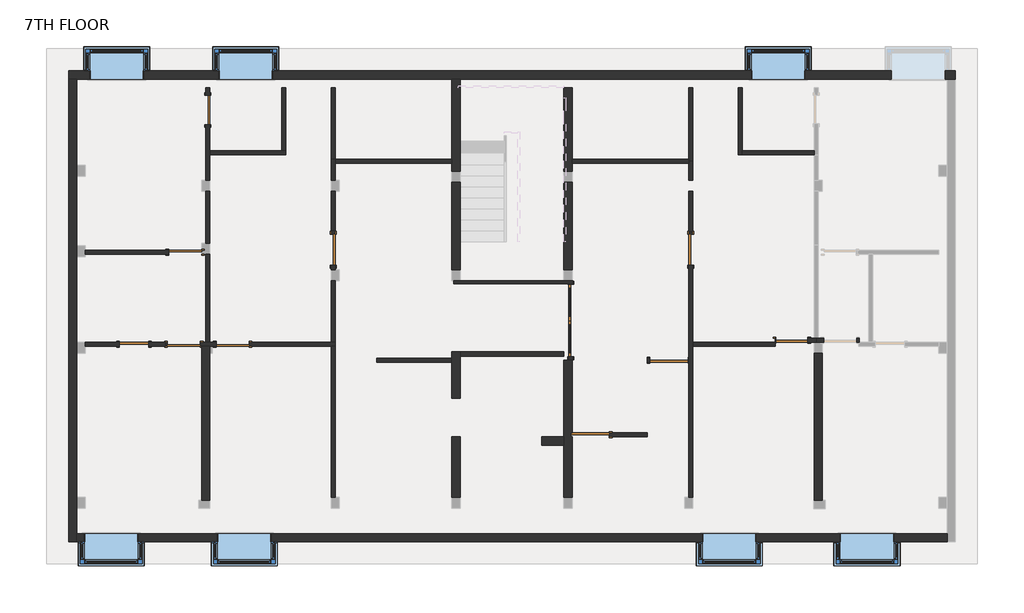
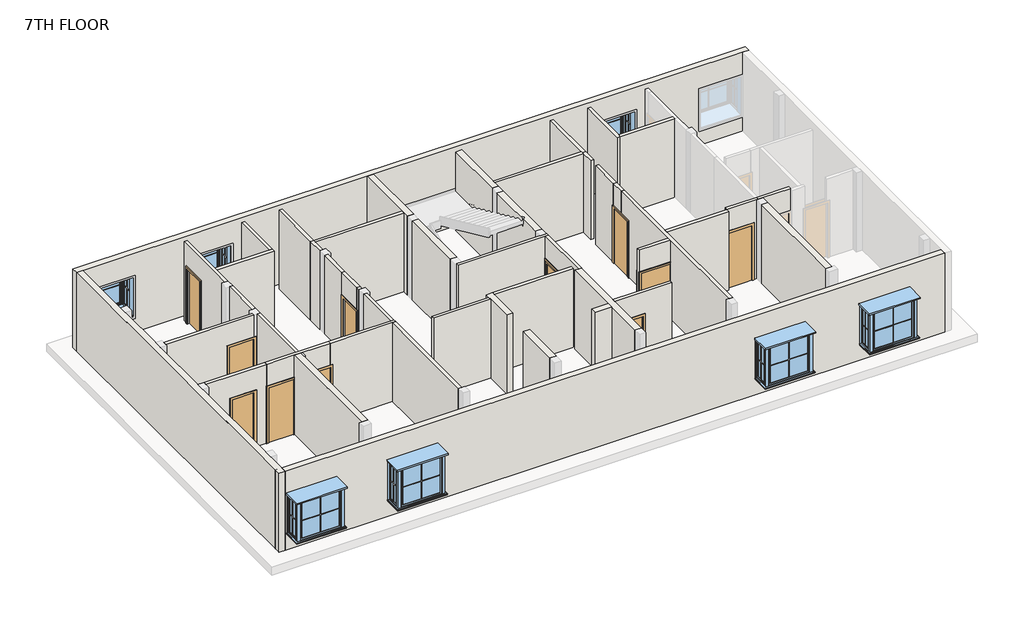
# One storey, part 1 of 2: 48 walls, 11 doors, 7 windows.
"""IFC4 building model written with IfcOpenShell, lengths in millimetres."""

from ifc_helpers import new_model, si_unit, frame, origin, place, context, project, spatial, polyline, outline, extrude, faceted_brep, transform, mapped, element, save
from components import door_04ab2522, m_door_single_panel_05506f71, door_07b5d71c, door_85b31ab1, door_1991e9a2, door_4c0a2014, door_82def9da, m_door_single_panel_3_x7_f8176753, m_door_single_panel_3_x7_ebb67e73, window_19bbd869

model = new_model("IFC4")

# Units and contexts
model_context = context("Model", 3, world=origin())
ifc_project = project(units=[si_unit("LENGTHUNIT", "METRE", prefix="MILLI")], contexts=[model_context])

# Site, building, storey
site = spatial("IfcSite", under=ifc_project)
building = spatial("IfcBuilding", under=site)
storey = spatial("IfcBuildingStorey", under=building, Name="7TH FLOOR", Elevation=25603.2)

# Doors
placement = place(None, origin())
door_shape = door_04ab2522(model_context)
element("IfcDoor", 1, ObjectType="M_Door-Double-Glass : 6'7\"X7'", at=placement, inside=storey, context=model_context, shape_type="MappedRepresentation", body=[
    mapped(door_shape, transform((1217.5394962, 1183.3817656, 25603.2), x_axis=(0.0, 1.0, 0.0), y_axis=(-1.0, 0.0, 0.0), z_axis=(0.0, 0.0, 1.0))),
])
m_door_single_panel_shape = m_door_single_panel_05506f71(model_context)
element("IfcDoor", 2, ObjectType="M_Door-Single-Panel", at=placement, inside=storey, context=model_context, shape_type="MappedRepresentation", body=[
    mapped(m_door_single_panel_shape, transform((1745.3012085, -1975.7432663, 25603.2), x_axis=(-1.0, 0.0, 0.0), y_axis=(0.0, -1.0, 0.0), z_axis=(0.0, 0.0, 1.0))),
])
element("IfcDoor", 3, ObjectType="M_Door-Single-Panel", at=placement, inside=storey, context=model_context, shape_type="MappedRepresentation", body=[
    mapped(m_door_single_panel_shape, transform((3933.4813133, 90.9578621, 25603.2), x_axis=(1.0, 0.0, 0.0), y_axis=(0.0, 1.0, 0.0), z_axis=(0.0, 0.0, 1.0))),
])
door_2_shape = door_07b5d71c(model_context)
element("IfcDoor", 4, ObjectType="M_Door-Single-Panel : 2'10\"X7' 2", at=placement, inside=storey, context=model_context, shape_type="MappedRepresentation", body=[
    mapped(door_2_shape, transform((-5360.3487995, 3142.9626891, 25603.2), x_axis=(0.0, -1.0, 0.0), y_axis=(1.0, 0.0, 0.0), z_axis=(0.0, 0.0, 1.0))),
])
door_3_shape = door_85b31ab1(model_context)
element("IfcDoor", 5, ObjectType="M_Door-Single-Panel : 2'10\"X7' 2", at=placement, inside=storey, context=model_context, shape_type="MappedRepresentation", body=[
    mapped(door_3_shape, transform((4532.9512082, 3142.9626891, 25603.2), x_axis=(0.0, -1.0, 0.0), y_axis=(1.0, 0.0, 0.0), z_axis=(0.0, 0.0, 1.0))),
])
door_4_shape = door_1991e9a2(model_context)
element("IfcDoor", 6, ObjectType="M_Door-Single-Panel : 2'11\"X7' 3", at=placement, inside=storey, context=model_context, shape_type="MappedRepresentation", body=[
    mapped(door_4_shape, transform((7330.1405552, 640.4567334, 25603.2), x_axis=(1.0, 0.0, 0.0), y_axis=(0.0, 1.0, 0.0), z_axis=(0.0, 0.0, 1.0))),
])
door_5_shape = door_4c0a2014(model_context)
element("IfcDoor", 7, ObjectType="M_Door-Single-Panel : 2'8\"X7'", at=placement, inside=storey, context=model_context, shape_type="MappedRepresentation", body=[
    mapped(door_5_shape, transform((-10873.4462614, 526.1567334, 25603.2), x_axis=(1.0, 0.0, 0.0), y_axis=(0.0, 1.0, 0.0), z_axis=(0.0, 0.0, 1.0))),
])
door_6_shape = door_82def9da(model_context)
element("IfcDoor", 8, ObjectType="M_Door-Single-Panel : 2'8\"X7'", at=placement, inside=storey, context=model_context, shape_type="MappedRepresentation", body=[
    mapped(door_6_shape, transform((-8827.4487992, 7008.6751452, 25603.2), x_axis=(0.0, 1.0, 0.0), y_axis=(-1.0, 0.0, 0.0), z_axis=(0.0, 0.0, 1.0))),
])
m_door_single_panel_3_x7_shape = m_door_single_panel_3_x7_f8176753(model_context)
element("IfcDoor", 9, ObjectType="M_Door-Single-Panel : 3'X7'", at=placement, inside=storey, context=model_context, shape_type="MappedRepresentation", body=[
    mapped(m_door_single_panel_3_x7_shape, transform((-9456.0987989, 3078.8567332, 25603.2), x_axis=(1.0, 0.0, 0.0), y_axis=(0.0, 1.0, 0.0), z_axis=(0.0, 0.0, 1.0))),
])
element("IfcDoor", 10, ObjectType="M_Door-Single-Panel : 3'X7'", at=placement, inside=storey, context=model_context, shape_type="MappedRepresentation", body=[
    mapped(m_door_single_panel_3_x7_shape, transform((-8144.8381465, 526.1567334, 25603.2), x_axis=(-1.0, 0.0, 0.0), y_axis=(0.0, -1.0, 0.0), z_axis=(0.0, 0.0, 1.0))),
])
m_door_single_panel_3_x7_2_shape = m_door_single_panel_3_x7_ebb67e73(model_context)
element("IfcDoor", 11, ObjectType="M_Door-Single-Panel : 3'X7'", at=placement, inside=storey, context=model_context, shape_type="MappedRepresentation", body=[
    mapped(m_door_single_panel_3_x7_2_shape, transform((-9494.1987992, 526.1567334, 25603.2), x_axis=(1.0, 0.0, 0.0), y_axis=(0.0, 1.0, 0.0), z_axis=(0.0, 0.0, 1.0))),
])

# Walls
element("IfcWall", 12, ObjectType="3.5\"", at=placement, inside=storey, context=model_context, shape_type="Brep", body=[
    faceted_brep([(-2020.2487998, 2196.2067742, 25603.2), (1158.0082462, 2196.2067742, 25603.2), (1272.3082462, 2196.2067742, 25603.2), (1272.3082462, 2196.2067742, 28651.2), (1158.0082462, 2196.2067742, 28651.2), (-2020.2487998, 2196.2067742, 28651.2), (-2020.2487998, 2285.1067742, 25603.2), (-2020.2487998, 2285.1067742, 28651.2), (-1845.5417538, 2285.1067742, 28651.2), (1024.6582462, 2285.1067742, 28651.2), (1253.2582462, 2285.1067742, 28651.2), (1272.3082462, 2285.1067742, 28651.2), (1272.3082462, 2285.1067742, 25603.2), (1253.2582462, 2285.1067742, 25603.2), (1024.6582462, 2285.1067742, 25603.2), (-1845.5417538, 2285.1067742, 25603.2)], [[[0, 1, 2, 3, 4, 5]], [[6, 7, 8, 9, 10, 11, 12, 13, 14, 15]], [[2, 1, 0, 6, 15, 14, 13, 12]], [[5, 4, 3, 11, 10, 9, 8, 7]], [[0, 5, 7, 6]], [[3, 2, 12, 11]]]),
])
element("IfcWall", 13, ObjectType="4.5\"", at=placement, inside=storey, context=model_context, shape_type="SweptSolid", body=[
    extrude(outline(polyline([(3132.0737955, 28651.2), (3628.3344162, 28651.2), (3628.3344162, 25603.2), (3574.7626891, 25603.2), (3574.7626891, 27736.8), (3132.0737955, 27736.8), (3132.0737955, 28651.2)])), frame((4475.8012082, 0.0, 0.0), z_axis=(1.0, 0.0, 0.0), x_axis=(0.0, 1.0, 0.0)), (0.0, 0.0, 1.0), 114.3),
])
element("IfcWall", 14, ObjectType="4.5\"", at=placement, inside=storey, context=model_context, shape_type="SweptSolid", body=[
    extrude(outline(polyline([(2711.1626891, 28651.2), (3671.8272228, 28651.2), (3671.8272228, 25603.2), (3574.7626891, 25603.2), (3574.7626891, 27736.8), (2711.1626891, 27736.8), (2711.1626891, 28651.2)])), frame((-5417.4987995, 0.0, 0.0), z_axis=(1.0, 0.0, 0.0), x_axis=(0.0, 1.0, 0.0)), (0.0, 0.0, 1.0), 114.3),
])
element("IfcWall", 15, ObjectType="4.5\"", at=placement, inside=storey, context=model_context, shape_type="Brep", body=[
    faceted_brep([(-7690.1644155, 469.0067334, 28651.2), (-8713.148796, 469.0067334, 28651.2), (-8771.750543, 469.0067334, 28651.2), (-9000.350543, 469.0067334, 28651.2), (-10009.8462614, 469.0067334, 28651.2), (-10009.8462614, 469.0067334, 25603.2), (-9951.3987992, 469.0067334, 25603.2), (-9951.3987992, 469.0067334, 27736.8), (-9036.9987992, 469.0067334, 27736.8), (-9036.9987992, 469.0067334, 25603.2), (-9000.350543, 469.0067334, 25603.2), (-8771.750543, 469.0067334, 25603.2), (-8713.148796, 469.0067334, 25603.2), (-8602.0381465, 469.0067334, 25603.2), (-8602.0381465, 469.0067334, 27736.8), (-7690.1644155, 469.0067334, 27736.8), (-10009.8462614, 583.3067334, 28651.2), (-7690.1644155, 583.3067334, 28651.2), (-7690.1644155, 583.3067334, 27736.8), (-8602.0381465, 583.3067334, 27736.8), (-8602.0381465, 583.3067334, 25603.2), (-9036.9987992, 583.3067334, 25603.2), (-9036.9987992, 583.3067334, 27736.8), (-9951.3987992, 583.3067334, 27736.8), (-9951.3987992, 583.3067334, 25603.2), (-10009.8462614, 583.3067334, 25603.2)], [[[0, 1, 2, 3, 4, 5, 6, 7, 8, 9, 10, 11, 12, 13, 14, 15]], [[16, 17, 18, 19, 20, 21, 22, 23, 24, 25]], [[5, 25, 24, 6]], [[9, 21, 20, 13, 12, 11, 10]], [[17, 0, 15, 18]], [[4, 3, 2, 1, 0, 17, 16]], [[5, 4, 16, 25]], [[8, 22, 21, 9]], [[7, 23, 22, 8]], [[23, 7, 6, 24]], [[19, 14, 13, 20]], [[14, 19, 18, 15]]]),
])
element("IfcWall", 16, ObjectType="4.5\"", at=placement, inside=storey, context=model_context, shape_type="Brep", body=[
    faceted_brep([(8000.0512079, 583.3067334, 25603.2), (8000.0512079, 583.3067334, 28651.2), (7942.9012047, 583.3067334, 28651.2), (6862.7668241, 583.3067334, 28651.2), (6862.7668241, 583.3067334, 25603.2), (6885.6405552, 583.3067334, 25603.2), (6885.6405552, 583.3067334, 27736.8), (7774.6405552, 583.3067334, 27736.8), (7774.6405552, 583.3067334, 25603.2), (7942.9012047, 583.3067334, 25603.2), (8000.0512079, 697.6067334, 28651.2), (8000.0512079, 697.6067334, 25603.2), (7942.9012079, 697.6067334, 25603.2), (7774.6405552, 697.6067334, 25603.2), (7774.6405552, 697.6067334, 27736.8), (6885.6405552, 697.6067334, 27736.8), (6885.6405552, 697.6067334, 25603.2), (6862.7668241, 697.6067334, 25603.2), (6862.7668241, 697.6067334, 28651.2), (7942.9012079, 697.6067334, 28651.2)], [[[0, 1, 2, 3, 4, 5, 6, 7, 8, 9]], [[10, 11, 12, 13, 14, 15, 16, 17, 18, 19]], [[4, 17, 16, 5]], [[11, 0, 9, 8, 13, 12]], [[1, 0, 11, 10]], [[3, 2, 1, 10, 19, 18]], [[4, 3, 18, 17]], [[7, 14, 13, 8]], [[14, 7, 6, 15]], [[15, 6, 5, 16]]]),
])
element("IfcWall", 17, ObjectType="4.5\"", at=placement, inside=storey, context=model_context, shape_type="Brep", body=[
    faceted_brep([(9187.5012047, 583.3067334, 25603.2), (9187.5012047, 583.3067334, 28651.2), (8171.5012047, 583.3067334, 28651.2), (8000.0512079, 583.3067334, 28651.2), (8000.0512079, 583.3067334, 25603.2), (8171.5012047, 583.3067334, 25603.2), (8209.6012079, 583.3067334, 25603.2), (8209.6012079, 583.3067334, 27736.8), (9124.0012079, 583.3067334, 27736.8), (9124.0012079, 583.3067334, 25603.2), (9187.5012047, 697.6067334, 28651.2), (9187.5012047, 697.6067334, 25603.2), (9124.0012079, 697.6067334, 25603.2), (9124.0012079, 697.6067334, 27736.8), (8209.6012079, 697.6067334, 27736.8), (8209.6012079, 697.6067334, 25603.2), (8057.2012079, 697.6067334, 25603.2), (8000.0512079, 697.6067334, 25603.2), (8000.0512079, 697.6067334, 28651.2), (8057.2012079, 697.6067334, 28651.2)], [[[0, 1, 2, 3, 4, 5, 6, 7, 8, 9]], [[10, 11, 12, 13, 14, 15, 16, 17, 18, 19]], [[11, 0, 9, 12]], [[4, 17, 16, 15, 6, 5]], [[1, 0, 11, 10]], [[3, 2, 1, 10, 19, 18]], [[4, 3, 18, 17]], [[7, 14, 13, 8]], [[8, 13, 12, 9]], [[14, 7, 6, 15]]]),
])
element("IfcWall", 18, ObjectType="4.5\"", at=placement, inside=storey, context=model_context, shape_type="SweptSolid", body=[
    extrude(outline(polyline([(25603.2, 3334.0114184), (28651.2, 3334.0114184), (28651.2, 1250.0012085), (27736.8, 1250.0012085), (27736.8, 2278.7012085), (25603.2, 2278.7012085), (25603.2, 3334.0114184)])), frame((0.0, -2032.8932663, 0.0), z_axis=(0.0, 1.0, 0.0), x_axis=(0.0, 0.0, 1.0)), (0.0, 0.0, 1.0), 114.3),
])
element("IfcWall", 19, ObjectType="4.5\"", at=placement, inside=storey, context=model_context, shape_type="SweptSolid", body=[
    extrude(outline(polyline([(27736.8, 4466.8813133), (25603.2, 4466.8813133), (25603.2, 4475.8012082), (28651.2, 4475.8012082), (28651.2, 3334.0114184), (25603.2, 3334.0114184), (25603.2, 3400.0813133), (27736.8, 3400.0813133), (27736.8, 4466.8813133)])), frame((0.0, 33.8078621, 0.0), z_axis=(0.0, 1.0, 0.0), x_axis=(0.0, 0.0, 1.0)), (0.0, 0.0, 1.0), 114.3),
])
element("IfcWall", 20, ObjectType="4.5\"", at=placement, inside=storey, context=model_context, shape_type="SweptSolid", body=[
    extrude(outline(polyline([(1021.4012085, 202.3067742), (-1848.7987998, 202.3067742), (-1848.7987998, 316.6067742), (1021.4012085, 316.6067742), (1021.4012085, 202.3067742)])), frame((0.0, 0.0, 25603.2), z_axis=(0.0, 0.0, 1.0), x_axis=(1.0, 0.0, 0.0)), (0.0, 0.0, 1.0), 3048.0),
])
element("IfcWall", 21, ObjectType="4.5\"", at=placement, inside=storey, context=model_context, shape_type="Brep", body=[
    faceted_brep([(1158.0082462, 2196.2067742, 25603.2), (1158.0082462, 2186.6817656, 25603.2), (1158.0082462, 2186.6817656, 27736.8), (1158.0082462, 180.0817656, 27736.8), (1158.0082462, 180.0817656, 25603.2), (1158.0082462, 90.9578621, 25603.2), (1158.0082462, 90.9578621, 28651.2), (1158.0082462, 2196.2067742, 28651.2), (1272.3082462, 2186.6817656, 27736.8), (1272.3082462, 2186.6817656, 25603.2), (1272.3082462, 2196.2067742, 25603.2), (1272.3082462, 2196.2067742, 28651.2), (1272.3082462, 90.9578621, 28651.2), (1272.3082462, 90.9578621, 25603.2), (1272.3082462, 180.0817656, 25603.2), (1272.3082462, 180.0817656, 27736.8), (1250.0012085, 90.9578621, 25603.2), (1250.0012085, 90.9578621, 28651.2)], [[[0, 1, 2, 3, 4, 5, 6, 7]], [[8, 9, 10, 11, 12, 13, 14, 15]], [[14, 13, 16, 5, 4]], [[10, 9, 1, 0]], [[6, 5, 16, 13, 12, 17]], [[7, 6, 17, 12, 11]], [[0, 7, 11, 10]], [[2, 1, 9, 8]], [[3, 2, 8, 15]], [[4, 3, 15, 14]]]),
])
element("IfcWall", 22, ObjectType="4.5\"", at=placement, inside=storey, context=model_context, shape_type="Brep", body=[
    faceted_brep([(1250.0012085, 5536.3067329, 25603.2), (4475.8012082, 5536.3067329, 25603.2), (4475.8012082, 5536.3067329, 28651.2), (1250.0012085, 5536.3067329, 28651.2), (1250.0012085, 5650.6067329, 25603.2), (1250.0012085, 5650.6067329, 28651.2), (4475.8012082, 5650.6067329, 28651.2), (4475.8012082, 5650.6067329, 25603.2), (4475.8012082, 5593.4567329, 25603.2), (4475.8012082, 5593.4567329, 28651.2)], [[[0, 1, 2, 3]], [[4, 5, 6, 7]], [[1, 0, 4, 7, 8]], [[3, 2, 9, 6, 5]], [[2, 1, 8, 7, 6, 9]], [[0, 3, 5, 4]]]),
])
element("IfcWall", 23, ObjectType="4.5\"", at=placement, inside=storey, context=model_context, shape_type="SweptSolid", body=[
    extrude(outline(polyline([(-5417.4987995, -3709.2932193), (-5417.4987995, 469.0067334), (-5303.1987995, 469.0067334), (-5303.1987995, -3709.2932193), (-5417.4987995, -3709.2932193)])), frame((0.0, 0.0, 25603.2), z_axis=(0.0, 0.0, 1.0), x_axis=(1.0, 0.0, 0.0)), (0.0, 0.0, 1.0), 3048.0),
])
element("IfcWall", 24, ObjectType="4.5\" 2", at=placement, inside=storey, context=model_context, shape_type="SweptSolid", body=[
    extrude(outline(polyline([(28651.2, -8998.8987989), (28651.2, -12224.6987989), (25603.2, -12224.6987989), (25603.2, -9913.2987989), (27736.8, -9913.2987989), (27736.8, -8998.8987989), (28651.2, -8998.8987989)])), frame((0.0, 3021.7067332, 0.0), z_axis=(0.0, 1.0, 0.0), x_axis=(0.0, 0.0, 1.0)), (0.0, 0.0, 1.0), 114.3),
])
element("IfcWall", 25, ObjectType="4.5\" 2", at=placement, inside=storey, context=model_context, shape_type="SweptSolid", body=[
    extrude(outline(polyline([(-8770.2987992, 4761.606733), (-8770.2987992, 3326.5067332), (-8884.5987992, 3326.5067332), (-8884.5987992, 4761.606733), (-8770.2987992, 4761.606733)])), frame((0.0, 0.0, 25603.2), z_axis=(0.0, 0.0, 1.0), x_axis=(1.0, 0.0, 0.0)), (0.0, 0.0, 1.0), 3048.0),
])
element("IfcWall", 26, ObjectType="4.5\" 2", at=placement, inside=storey, context=model_context, shape_type="Brep", body=[
    faceted_brep([(-8770.2987992, 7415.0751452, 27736.8), (-8770.2987992, 7415.0751452, 25603.2), (-8770.2987992, 7631.8067329, 25603.2), (-8770.2987992, 7631.8067329, 28651.2), (-8770.2987992, 5879.2067329, 28651.2), (-8770.2987992, 5764.9067329, 28651.2), (-8770.2987992, 5066.406733, 28651.2), (-8770.2987992, 5066.406733, 25603.2), (-8770.2987992, 5764.9067329, 25603.2), (-8770.2987992, 5879.2067329, 25603.2), (-8770.2987992, 6602.2751452, 25603.2), (-8770.2987992, 6602.2751452, 27736.8), (-8884.5987992, 7631.8067329, 25603.2), (-8884.5987992, 7415.0751452, 25603.2), (-8884.5987992, 7415.0751452, 27736.8), (-8884.5987992, 6602.2751452, 27736.8), (-8884.5987992, 6602.2751452, 25603.2), (-8884.5987992, 5066.406733, 25603.2), (-8884.5987992, 5066.406733, 28651.2), (-8884.5987992, 7631.8067329, 28651.2)], [[[0, 1, 2, 3, 4, 5, 6, 7, 8, 9, 10, 11]], [[12, 13, 14, 15, 16, 17, 18, 19]], [[2, 1, 13, 12]], [[10, 9, 8, 7, 17, 16]], [[3, 2, 12, 19]], [[6, 5, 4, 3, 19, 18]], [[7, 6, 18, 17]], [[14, 13, 1, 0]], [[15, 14, 0, 11]], [[16, 15, 11, 10]]]),
])
element("IfcWall", 27, ObjectType="4.5\" 2", at=placement, inside=storey, context=model_context, shape_type="Brep", body=[
    faceted_brep([(-8770.2987992, 5764.9067329, 25603.2), (-6674.7987994, 5764.9067329, 25603.2), (-6674.7987994, 5764.9067329, 28651.2), (-8770.2987992, 5764.9067329, 28651.2), (-8770.2987992, 5879.2067329, 25603.2), (-8770.2987992, 5879.2067329, 28651.2), (-6789.0987994, 5879.2067329, 28651.2), (-6674.7987994, 5879.2067329, 28651.2), (-6674.7987994, 5879.2067329, 25603.2), (-6789.0987994, 5879.2067329, 25603.2)], [[[0, 1, 2, 3]], [[4, 5, 6, 7, 8, 9]], [[1, 0, 4, 9, 8]], [[3, 2, 7, 6, 5]], [[0, 3, 5, 4]], [[2, 1, 8, 7]]]),
])
element("IfcWall", 28, ObjectType="4.5\" 2", at=placement, inside=storey, context=model_context, shape_type="SweptSolid", body=[
    extrude(outline(polyline([(-6674.7987994, 7631.8067329), (-6674.7987994, 5879.2067329), (-6789.0987994, 5879.2067329), (-6789.0987994, 7631.8067329), (-6674.7987994, 7631.8067329)])), frame((0.0, 0.0, 25603.2), z_axis=(0.0, 0.0, 1.0), x_axis=(1.0, 0.0, 0.0)), (0.0, 0.0, 1.0), 3048.0),
])
element("IfcWall", 29, ObjectType="4.5\" 2", at=placement, inside=storey, context=model_context, shape_type="SweptSolid", body=[
    extrude(outline(polyline([(27736.8, -10467.0462614), (25603.2, -10467.0462614), (25603.2, -10009.8462614), (28651.2, -10009.8462614), (28651.2, -12224.6987989), (25603.2, -12224.6987989), (25603.2, -11279.8462614), (27736.8, -11279.8462614), (27736.8, -10467.0462614)])), frame((0.0, 469.0067334, 0.0), z_axis=(0.0, 1.0, 0.0), x_axis=(0.0, 0.0, 1.0)), (0.0, 0.0, 1.0), 114.3),
])
element("IfcWall", 30, ObjectType="4.5\" 2", at=placement, inside=storey, context=model_context, shape_type="SweptSolid", body=[
    extrude(outline(polyline([(-8770.298796, 3021.7067332), (-8770.298796, 583.3067804), (-8884.598796, 583.3067804), (-8884.598796, 3021.7067332), (-8770.298796, 3021.7067332)])), frame((0.0, 0.0, 25603.2), z_axis=(0.0, 0.0, 1.0), x_axis=(1.0, 0.0, 0.0)), (0.0, 0.0, 1.0), 3048.0),
])
element("IfcWall", 31, ObjectType="4.5\" 2", at=placement, inside=storey, context=model_context, shape_type="Brep", body=[
    faceted_brep([(-5303.1987995, 469.0067334, 28651.2), (-5417.4987995, 469.0067334, 28651.2), (-7690.1644155, 469.0067334, 28651.2), (-7690.1644155, 469.0067334, 27736.8), (-7687.6381465, 469.0067334, 27736.8), (-7687.6381465, 469.0067334, 25603.2), (-5417.4987995, 469.0067334, 25603.2), (-5303.1987995, 469.0067334, 25603.2), (-7690.1644155, 583.3067334, 28651.2), (-5417.4987995, 583.3067334, 28651.2), (-5303.1987995, 583.3067334, 28651.2), (-5303.1987995, 583.3067334, 25603.2), (-5417.4987995, 583.3067334, 25603.2), (-7687.6381465, 583.3067334, 25603.2), (-7687.6381465, 583.3067334, 27736.8), (-7690.1644155, 583.3067334, 27736.8)], [[[0, 1, 2, 3, 4, 5, 6, 7]], [[8, 9, 10, 11, 12, 13, 14, 15]], [[11, 7, 6, 5, 13, 12]], [[2, 1, 0, 10, 9, 8]], [[2, 8, 15, 3]], [[0, 7, 11, 10]], [[14, 4, 3, 15]], [[4, 14, 13, 5]]]),
])
element("IfcWall", 32, ObjectType="4.5\" 2", at=placement, inside=storey, context=model_context, shape_type="SweptSolid", body=[
    extrude(outline(polyline([(-5303.1987995, 2285.1067802), (-5303.1987995, 583.3067334), (-5417.4987995, 583.3067334), (-5417.4987995, 2285.1067802), (-5303.1987995, 2285.1067802)])), frame((0.0, 0.0, 25603.2), z_axis=(0.0, 0.0, 1.0), x_axis=(1.0, 0.0, 0.0)), (0.0, 0.0, 1.0), 3048.0),
])
element("IfcWall", 33, ObjectType="4.5\" 2", at=placement, inside=storey, context=model_context, shape_type="Brep", body=[
    faceted_brep([(-5303.1987995, 2589.9067802, 25603.2), (-5303.1987995, 2711.1626891, 25603.2), (-5303.1987995, 2711.1626891, 27736.8), (-5303.1987995, 2711.1626891, 28651.2), (-5303.1987995, 2589.9067802, 28651.2), (-5417.4987995, 2589.9067802, 25603.2), (-5417.4987995, 2589.9067802, 28651.2), (-5417.4987995, 2711.1626891, 28651.2), (-5417.4987995, 2711.1626891, 27736.8), (-5417.4987995, 2711.1626891, 25603.2)], [[[0, 1, 2, 3, 4]], [[5, 6, 7, 8, 9]], [[1, 0, 5, 9]], [[3, 2, 1, 9, 8, 7]], [[4, 3, 7, 6]], [[0, 4, 6, 5]]]),
])
element("IfcWall", 34, ObjectType="4.5\" 2", at=placement, inside=storey, context=model_context, shape_type="SweptSolid", body=[
    extrude(outline(polyline([(-5303.1987995, 4761.606733), (-5303.1987995, 3671.8272228), (-5417.4987995, 3671.8272228), (-5417.4987995, 4761.606733), (-5303.1987995, 4761.606733)])), frame((0.0, 0.0, 25603.2), z_axis=(0.0, 0.0, 1.0), x_axis=(1.0, 0.0, 0.0)), (0.0, 0.0, 1.0), 3048.0),
])
element("IfcWall", 35, ObjectType="4.5\" 2", at=placement, inside=storey, context=model_context, shape_type="Brep", body=[
    faceted_brep([(-5303.1987995, 5066.406733, 25603.2), (-5303.1987995, 5536.3067329, 25603.2), (-5303.1987995, 5650.6067329, 25603.2), (-5303.1987995, 5650.6067329, 28651.2), (-5303.1987995, 5536.3067329, 28651.2), (-5303.1987995, 5066.406733, 28651.2), (-5417.4987995, 5066.406733, 25603.2), (-5417.4987995, 5066.406733, 28651.2), (-5417.4987995, 5650.6067329, 28651.2), (-5417.4987995, 5650.6067329, 25603.2)], [[[0, 1, 2, 3, 4, 5]], [[6, 7, 8, 9]], [[2, 1, 0, 6, 9]], [[5, 4, 3, 8, 7]], [[0, 5, 7, 6]], [[3, 2, 9, 8]]]),
])
element("IfcWall", 36, ObjectType="4.5\" 2", at=placement, inside=storey, context=model_context, shape_type="SweptSolid", body=[
    extrude(outline(polyline([(-2077.3987998, 5536.3067329), (-5303.1987995, 5536.3067329), (-5303.1987995, 5650.6067329), (-2077.3987998, 5650.6067329), (-2077.3987998, 5536.3067329)])), frame((0.0, 0.0, 25603.2), z_axis=(0.0, 0.0, 1.0), x_axis=(1.0, 0.0, 0.0)), (0.0, 0.0, 1.0), 3048.0),
])
element("IfcWall", 37, ObjectType="4.5\" 2", at=placement, inside=storey, context=model_context, shape_type="SweptSolid", body=[
    extrude(outline(polyline([(-5417.4987995, 5650.6067329), (-5417.4987995, 7631.8067329), (-5303.1987995, 7631.8067329), (-5303.1987995, 5650.6067329), (-5417.4987995, 5650.6067329)])), frame((0.0, 0.0, 25603.2), z_axis=(0.0, 0.0, 1.0), x_axis=(1.0, 0.0, 0.0)), (0.0, 0.0, 1.0), 3048.0),
])
element("IfcWall", 38, ObjectType="4.5\" 2", at=placement, inside=storey, context=model_context, shape_type="Brep", body=[
    faceted_brep([(4475.8012082, 5593.4567329, 25603.2), (4475.8012082, 5536.3067329, 25603.2), (4475.8012082, 5066.40678, 25603.2), (4475.8012082, 5066.40678, 28651.2), (4475.8012082, 5536.3067329, 28651.2), (4475.8012082, 5593.4567329, 28651.2), (4590.1012082, 5593.4567329, 25603.2), (4590.1012082, 5593.4567329, 28651.2), (4590.1012082, 5066.40678, 28651.2), (4590.1012082, 5066.40678, 25603.2)], [[[0, 1, 2, 3, 4, 5]], [[6, 7, 8, 9]], [[2, 1, 0, 6, 9]], [[3, 2, 9, 8]], [[5, 4, 3, 8, 7]], [[0, 5, 7, 6]]]),
])
element("IfcWall", 39, ObjectType="4.5\" 2", at=placement, inside=storey, context=model_context, shape_type="SweptSolid", body=[
    extrude(outline(polyline([(4475.8012082, 3628.3344162), (4475.8012082, 4761.606733), (4590.1012082, 4761.606733), (4590.1012082, 3628.3344162), (4475.8012082, 3628.3344162)])), frame((0.0, 0.0, 25603.2), z_axis=(0.0, 0.0, 1.0), x_axis=(1.0, 0.0, 0.0)), (0.0, 0.0, 1.0), 3048.0),
])
element("IfcWall", 40, ObjectType="4.5\" 2", at=placement, inside=storey, context=model_context, shape_type="Brep", body=[
    faceted_brep([(4475.8012082, -3709.2932193, 25603.2), (4475.8012082, -3709.2932193, 28651.2), (4475.8012082, 33.8078621, 28651.2), (4475.8012082, 148.1078621, 28651.2), (4475.8012082, 3132.0737955, 28651.2), (4475.8012082, 3132.0737955, 27736.8), (4475.8012082, 2711.1626891, 27736.8), (4475.8012082, 2711.1626891, 25603.2), (4475.8012082, 148.1078621, 25603.2), (4475.8012082, 33.8078621, 25603.2), (4590.1012082, -3709.2932193, 28651.2), (4590.1012082, -3709.2932193, 25603.2), (4590.1012082, 469.0067334, 25603.2), (4590.1012082, 583.3067334, 25603.2), (4590.1012082, 2711.1626891, 25603.2), (4590.1012082, 2711.1626891, 27736.8), (4590.1012082, 3132.0737955, 27736.8), (4590.1012082, 3132.0737955, 28651.2), (4590.1012082, 583.3067334, 28651.2), (4590.1012082, 469.0067334, 28651.2)], [[[0, 1, 2, 3, 4, 5, 6, 7, 8, 9]], [[10, 11, 12, 13, 14, 15, 16, 17, 18, 19]], [[11, 0, 9, 8, 7, 14, 13, 12]], [[1, 0, 11, 10]], [[4, 3, 2, 1, 10, 19, 18, 17]], [[4, 17, 16, 5]], [[6, 15, 14, 7]], [[15, 6, 5, 16]]]),
])
element("IfcWall", 41, ObjectType="4.5\" 2", at=placement, inside=storey, context=model_context, shape_type="SweptSolid", body=[
    extrude(outline(polyline([(6862.7668241, 469.0067334), (4590.1012082, 469.0067334), (4590.1012082, 583.3067334), (6862.7668241, 583.3067334), (6862.7668241, 469.0067334)])), frame((0.0, 0.0, 25603.2), z_axis=(0.0, 0.0, 1.0), x_axis=(1.0, 0.0, 0.0)), (0.0, 0.0, 1.0), 3048.0),
])
element("IfcWall", 42, ObjectType="4.5\" 2", at=placement, inside=storey, context=model_context, shape_type="Brep", body=[
    faceted_brep([(4590.1012082, 5593.4567329, 25603.2), (4590.1012082, 7631.8067329, 25603.2), (4590.1012082, 7631.8067329, 28651.2), (4590.1012082, 5593.4567329, 28651.2), (4475.8012082, 5593.4567329, 25603.2), (4475.8012082, 5593.4567329, 28651.2), (4475.8012082, 5650.6067329, 28651.2), (4475.8012082, 7631.8067329, 28651.2), (4475.8012082, 7631.8067329, 25603.2), (4475.8012082, 5650.6067329, 25603.2)], [[[0, 1, 2, 3]], [[4, 5, 6, 7, 8, 9]], [[1, 0, 4, 9, 8]], [[2, 1, 8, 7]], [[3, 2, 7, 6, 5]], [[0, 3, 5, 4]]]),
])
element("IfcWall", 43, ObjectType="4.5\" 2", at=placement, inside=storey, context=model_context, shape_type="Brep", body=[
    faceted_brep([(5847.401208, 7631.8067329, 25603.2), (5847.401208, 5764.9067329, 25603.2), (5847.401208, 5764.9067329, 28651.2), (5847.401208, 7631.8067329, 28651.2), (5961.701208, 7631.8067329, 25603.2), (5961.701208, 7631.8067329, 28651.2), (5961.701208, 5879.2067329, 28651.2), (5961.701208, 5764.9067329, 28651.2), (5961.701208, 5764.9067329, 25603.2), (5961.701208, 5879.2067329, 25603.2)], [[[0, 1, 2, 3]], [[4, 5, 6, 7, 8, 9]], [[1, 0, 4, 9, 8]], [[3, 2, 7, 6, 5]], [[0, 3, 5, 4]], [[2, 1, 8, 7]]]),
])
element("IfcWall", 44, ObjectType="4.5\" 2", at=placement, inside=storey, context=model_context, shape_type="SweptSolid", body=[
    extrude(outline(polyline([(7942.9012079, 5764.9067329), (5961.701208, 5764.9067329), (5961.701208, 5879.2067329), (7942.9012079, 5879.2067329), (7942.9012079, 5764.9067329)])), frame((0.0, 0.0, 25603.2), z_axis=(0.0, 0.0, 1.0), x_axis=(1.0, 0.0, 0.0)), (0.0, 0.0, 1.0), 3048.0),
])
element("IfcWall", 45, ObjectType="4.5\" 2", at=placement, inside=storey, context=model_context, shape_type="SweptSolid", body=[
    extrude(outline(polyline([(-2077.3987998, 33.8078621), (-4161.4090098, 33.8078621), (-4161.4090098, 148.1078621), (-2077.3987998, 148.1078621), (-2077.3987998, 33.8078621)])), frame((0.0, 0.0, 25603.2), z_axis=(0.0, 0.0, 1.0), x_axis=(1.0, 0.0, 0.0)), (0.0, 0.0, 1.0), 3048.0),
])
element("IfcWall", 46, ObjectType="9\"", at=placement, inside=storey, context=model_context, shape_type="Brep", body=[
    faceted_brep([(-12681.8987957, 7860.4067329, 25603.2), (-12453.2987957, 7860.4067329, 25603.2), (-2074.1417538, 7860.4067329, 25603.2), (-1845.5417538, 7860.4067329, 25603.2), (11625.9012075, 7860.4067329, 25603.2), (11854.5012075, 7860.4067329, 25603.2), (11854.5012075, 7860.4067329, 28651.2), (11625.9012075, 7860.4067329, 28651.2), (-1845.5417538, 7860.4067329, 28651.2), (-2074.1417538, 7860.4067329, 28651.2), (-12453.2987957, 7860.4067329, 28651.2), (-12681.8987957, 7860.4067329, 28651.2), (11575.8012075, 7860.4067329, 27754.0), (11575.8012075, 7860.4067329, 26203.2), (10075.8012075, 7860.4067329, 26203.2), (10075.8012075, 7860.4067329, 27754.0), (7702.301208, 7860.4067329, 27754.0), (7702.301208, 7860.4067329, 26203.2), (6202.301208, 7860.4067329, 26203.2), (6202.301208, 7860.4067329, 27754.0), (-7029.6987993, 7860.4067329, 27754.0), (-7029.6987993, 7860.4067329, 26203.2), (-8529.6987993, 7860.4067329, 26203.2), (-8529.6987993, 7860.4067329, 27754.0), (-10598.3987957, 7860.4067329, 27754.0), (-10598.3987957, 7860.4067329, 26203.2), (-12098.3987957, 7860.4067329, 26203.2), (-12098.3987957, 7860.4067329, 27754.0), (-12681.8987957, 8089.0067329, 25603.2), (-12681.8987957, 8089.0067329, 28651.2), (11854.5012075, 8089.0067329, 28651.2), (11854.5012075, 8089.0067329, 25603.2), (11575.8012075, 8089.0067329, 27754.0), (10075.8012075, 8089.0067329, 27754.0), (10075.8012075, 8089.0067329, 26203.2), (11575.8012075, 8089.0067329, 26203.2), (7702.301208, 8089.0067329, 27754.0), (6202.301208, 8089.0067329, 27754.0), (6202.301208, 8089.0067329, 26203.2), (7702.301208, 8089.0067329, 26203.2), (-7029.6987993, 8089.0067329, 27754.0), (-8529.6987993, 8089.0067329, 27754.0), (-8529.6987993, 8089.0067329, 26203.2), (-7029.6987993, 8089.0067329, 26203.2), (-10598.3987957, 8089.0067329, 27754.0), (-12098.3987957, 8089.0067329, 27754.0), (-12098.3987957, 8089.0067329, 26203.2), (-10598.3987957, 8089.0067329, 26203.2)], [[[0, 1, 2, 3, 4, 5, 6, 7, 8, 9, 10, 11], [12, 13, 14, 15], [16, 17, 18, 19], [20, 21, 22, 23], [24, 25, 26, 27]], [[28, 29, 30, 31], [32, 33, 34, 35], [36, 37, 38, 39], [40, 41, 42, 43], [44, 45, 46, 47]], [[5, 4, 3, 2, 1, 0, 28, 31]], [[11, 10, 9, 8, 7, 6, 30, 29]], [[6, 5, 31, 30]], [[0, 11, 29, 28]], [[13, 12, 32, 35]], [[14, 13, 35, 34]], [[15, 14, 34, 33]], [[12, 15, 33, 32]], [[17, 16, 36, 39]], [[18, 17, 39, 38]], [[19, 18, 38, 37]], [[16, 19, 37, 36]], [[21, 20, 40, 43]], [[22, 21, 43, 42]], [[23, 22, 42, 41]], [[20, 23, 41, 40]], [[25, 24, 44, 47]], [[26, 25, 47, 46]], [[27, 26, 46, 45]], [[24, 27, 45, 44]]]),
])
element("IfcWall", 47, ObjectType="9\"", at=placement, inside=storey, context=model_context, shape_type="Brep", body=[
    faceted_brep([(-12453.2987957, -4941.1932661, 25603.2), (-12453.2987957, -4712.5932661, 25603.2), (-12453.2987957, -4014.0932671, 25603.2), (-12453.2987957, -3709.2932671, 25603.2), (-12453.2987957, 278.5067334, 25603.2), (-12453.2987957, 583.3067334, 25603.2), (-12453.2987957, 2951.8567332, 25603.2), (-12453.2987957, 3256.6567332, 25603.2), (-12453.2987957, 5174.3567339, 25603.2), (-12453.2987957, 5479.1567339, 25603.2), (-12453.2987957, 7860.4067329, 25603.2), (-12453.2987957, 7860.4067329, 28651.2), (-12453.2987957, 5479.1567339, 28651.2), (-12453.2987957, 5174.3567339, 28651.2), (-12453.2987957, 3256.6567332, 28651.2), (-12453.2987957, 2951.8567332, 28651.2), (-12453.2987957, 583.3067334, 28651.2), (-12453.2987957, 278.5067334, 28651.2), (-12453.2987957, -3709.2932671, 28651.2), (-12453.2987957, -4014.0932671, 28651.2), (-12453.2987957, -4712.5932661, 28651.2), (-12453.2987957, -4941.1932661, 28651.2), (-12681.8987957, -4941.1932661, 25603.2), (-12681.8987957, -4941.1932661, 28651.2), (-12681.8987957, 7860.4067329, 28651.2), (-12681.8987957, 7860.4067329, 25603.2)], [[[0, 1, 2, 3, 4, 5, 6, 7, 8, 9, 10, 11, 12, 13, 14, 15, 16, 17, 18, 19, 20, 21]], [[22, 23, 24, 25]], [[10, 9, 8, 7, 6, 5, 4, 3, 2, 1, 0, 22, 25]], [[21, 20, 19, 18, 17, 16, 15, 14, 13, 12, 11, 24, 23]], [[11, 10, 25, 24]], [[0, 21, 23, 22]]]),
])
element("IfcWall", 48, ObjectType="9\"", at=placement, inside=storey, context=model_context, shape_type="Brep", body=[
    faceted_brep([(-12453.2987957, -4712.5932661, 25603.2), (-12453.2987957, -4014.0932671, 25603.2), (-12453.2987957, -3709.2932671, 25603.2), (-12453.2987957, 278.5067334, 25603.2), (-12453.2987957, 583.3067334, 25603.2), (-12453.2987957, 2951.8567332, 25603.2), (-12453.2987957, 3256.6567332, 25603.2), (-12453.2987957, 5174.3567339, 25603.2), (-12453.2987957, 5479.1567339, 25603.2), (-12453.2987957, 7860.4067329, 25603.2), (-12453.2987957, 7860.4067329, 28651.2), (-12453.2987957, 5479.1567339, 28651.2), (-12453.2987957, 5174.3567339, 28651.2), (-12453.2987957, 3256.6567332, 28651.2), (-12453.2987957, 2951.8567332, 28651.2), (-12453.2987957, 583.3067334, 28651.2), (-12453.2987957, 278.5067334, 28651.2), (-12453.2987957, -3709.2932671, 28651.2), (-12453.2987957, -4014.0932671, 28651.2), (-12453.2987957, -4712.5932661, 28651.2), (-12681.8987957, -4712.5932661, 25603.2), (-12681.8987957, -4712.5932661, 28651.2), (-12681.8987957, 7860.4067329, 28651.2), (-12681.8987957, 7860.4067329, 25603.2)], [[[0, 1, 2, 3, 4, 5, 6, 7, 8, 9, 10, 11, 12, 13, 14, 15, 16, 17, 18, 19]], [[20, 21, 22, 23]], [[9, 8, 7, 6, 5, 4, 3, 2, 1, 0, 20, 23]], [[19, 18, 17, 16, 15, 14, 13, 12, 11, 10, 22, 21]], [[10, 9, 23, 22]], [[0, 19, 21, 20]]]),
])
element("IfcWall", 49, ObjectType="9\"", at=placement, inside=storey, context=model_context, shape_type="Brep", body=[
    faceted_brep([(-9000.350543, 469.0067334, 25603.2), (-9000.350543, -3785.4932196, 25603.2), (-9000.350543, -3785.4932196, 28651.2), (-9000.350543, 469.0067334, 28651.2), (-8771.750543, 469.0067334, 25603.2), (-8771.750543, 469.0067334, 28651.2), (-8771.750543, 278.5067334, 28651.2), (-8771.750543, -3785.4932196, 28651.2), (-8771.750543, -3785.4932196, 25603.2), (-8771.750543, 278.5067334, 25603.2)], [[[0, 1, 2, 3]], [[4, 5, 6, 7, 8, 9]], [[1, 0, 4, 9, 8]], [[2, 1, 8, 7]], [[3, 2, 7, 6, 5]], [[0, 3, 5, 4]]]),
])
element("IfcWall", 50, ObjectType="9\"", at=placement, inside=storey, context=model_context, shape_type="Brep", body=[
    faceted_brep([(-2077.3987998, 316.6067742, 25603.2), (-2077.3987998, 148.1078621, 25603.2), (-2077.3987998, 33.8078621, 25603.2), (-2077.3987998, -972.2341552, 25603.2), (-2077.3987998, -972.2341552, 28651.2), (-2077.3987998, 33.8078621, 28651.2), (-2077.3987998, 148.1078621, 28651.2), (-2077.3987998, 316.6067742, 28651.2), (-1848.7987998, 316.6067742, 25603.2), (-1848.7987998, 316.6067742, 28651.2), (-1848.7987998, 202.3067742, 28651.2), (-1848.7987998, -972.2341552, 28651.2), (-1848.7987998, -972.2341552, 25603.2), (-1848.7987998, 202.3067742, 25603.2)], [[[0, 1, 2, 3, 4, 5, 6, 7]], [[8, 9, 10, 11, 12, 13]], [[3, 2, 1, 0, 8, 13, 12]], [[4, 3, 12, 11]], [[7, 6, 5, 4, 11, 10, 9]], [[0, 7, 9, 8]]]),
])
element("IfcWall", 51, ObjectType="9\"", at=placement, inside=storey, context=model_context, shape_type="SweptSolid", body=[
    extrude(outline(polyline([(-2077.3987998, -3709.2932663), (-2077.3987998, -2032.8932663), (-1848.7987998, -2032.8932663), (-1848.7987998, -3709.2932663), (-2077.3987998, -3709.2932663)])), frame((0.0, 0.0, 25603.2), z_axis=(0.0, 0.0, 1.0), x_axis=(1.0, 0.0, 0.0)), (0.0, 0.0, 1.0), 3048.0),
])
element("IfcWall", 52, ObjectType="9\"", at=placement, inside=storey, context=model_context, shape_type="SweptSolid", body=[
    extrude(outline(polyline([(1021.4012085, -2261.4932663), (412.152227, -2261.4932663), (412.152227, -2032.8932663), (1021.4012085, -2032.8932663), (1021.4012085, -2261.4932663)])), frame((0.0, 0.0, 25603.2), z_axis=(0.0, 0.0, 1.0), x_axis=(1.0, 0.0, 0.0)), (0.0, 0.0, 1.0), 3048.0),
])
element("IfcWall", 53, ObjectType="9\"", at=placement, inside=storey, context=model_context, shape_type="Brep", body=[
    faceted_brep([(1021.4012085, 90.9578621, 25603.2), (1021.4012085, -2032.8932663, 25603.2), (1021.4012085, -2261.4932663, 25603.2), (1021.4012085, -3709.2932193, 25603.2), (1021.4012085, -3709.2932193, 28651.2), (1021.4012085, -2261.4932663, 28651.2), (1021.4012085, -2032.8932663, 28651.2), (1021.4012085, 90.9578621, 28651.2), (1250.0012085, -3709.2932193, 28651.2), (1250.0012085, -3709.2932193, 25603.2), (1250.0012085, -2032.8932663, 25603.2), (1250.0012085, -2032.8932663, 27736.8), (1250.0012085, -1918.5932663, 27736.8), (1250.0012085, -1918.5932663, 25603.2), (1250.0012085, 90.9578621, 25603.2), (1250.0012085, 90.9578621, 28651.2), (1250.0012085, -1918.5932663, 28651.2), (1250.0012085, -2032.8932663, 28651.2), (1158.0082462, 90.9578621, 25603.2), (1211.9012085, -1918.5932663, 25603.2), (1211.9012085, -2032.8932663, 25603.2), (1158.0082462, 90.9578621, 28651.2), (1211.9012085, -1918.5932663, 27736.8), (1211.9012085, -2032.8932663, 27736.8)], [[[0, 1, 2, 3, 4, 5, 6, 7]], [[8, 9, 10, 11, 12, 13, 14, 15, 16, 17]], [[3, 2, 1, 0, 18, 14, 13, 19, 20, 10, 9]], [[4, 3, 9, 8]], [[7, 6, 5, 4, 8, 17, 16, 15, 21]], [[0, 7, 21, 15, 14, 18]], [[22, 19, 13, 12]], [[20, 23, 11, 10]], [[19, 22, 23, 20]], [[23, 22, 12, 11]]]),
])
element("IfcWall", 54, ObjectType="9\"", at=placement, inside=storey, context=model_context, shape_type="SweptSolid", body=[
    extrude(outline(polyline([(-2074.1417538, 5320.4067329), (-2074.1417538, 7860.4067329), (-1845.5417538, 7860.4067329), (-1845.5417538, 5320.4067329), (-2074.1417538, 5320.4067329)])), frame((0.0, 0.0, 25603.2), z_axis=(0.0, 0.0, 1.0), x_axis=(1.0, 0.0, 0.0)), (0.0, 0.0, 1.0), 3048.0),
])
element("IfcWall", 55, ObjectType="9\"", at=placement, inside=storey, context=model_context, shape_type="SweptSolid", body=[
    extrude(outline(polyline([(-2074.1417538, 2589.906774), (-2074.1417538, 5015.606774), (-1845.5417538, 5015.606774), (-1845.5417538, 2589.906774), (-2074.1417538, 2589.906774)])), frame((0.0, 0.0, 25603.2), z_axis=(0.0, 0.0, 1.0), x_axis=(1.0, 0.0, 0.0)), (0.0, 0.0, 1.0), 3048.0),
])
element("IfcWall", 56, ObjectType="9\"", at=placement, inside=storey, context=model_context, shape_type="Brep", body=[
    faceted_brep([(1021.4012085, 7631.8067329, 25603.2), (1021.4012085, 5320.4067329, 25603.2), (1021.4012085, 5320.4067329, 28651.2), (1021.4012085, 7631.8067329, 28651.2), (1250.0012085, 7631.8067329, 25603.2), (1250.0012085, 7631.8067329, 28651.2), (1250.0012085, 5650.6067329, 28651.2), (1250.0012085, 5536.3067329, 28651.2), (1250.0012085, 5320.4067329, 28651.2), (1250.0012085, 5320.4067329, 25603.2), (1250.0012085, 5536.3067329, 25603.2), (1250.0012085, 5650.6067329, 25603.2)], [[[0, 1, 2, 3]], [[4, 5, 6, 7, 8, 9, 10, 11]], [[1, 0, 4, 11, 10, 9]], [[2, 1, 9, 8]], [[3, 2, 8, 7, 6, 5]], [[0, 3, 5, 4]]]),
])
element("IfcWall", 57, ObjectType="9\"", at=placement, inside=storey, context=model_context, shape_type="Brep", body=[
    faceted_brep([(1021.4012085, 5015.6067329, 25603.2), (1021.4012085, 2589.9067742, 25603.2), (1021.4012085, 2589.9067742, 28651.2), (1021.4012085, 5015.6067329, 28651.2), (1250.0012085, 5015.6067329, 25603.2), (1250.0012085, 5015.6067329, 28651.2), (1250.0012085, 2589.9067742, 28651.2), (1250.0012085, 2589.9067742, 25603.2), (1024.6582462, 2589.9067742, 25603.2), (1024.6582462, 2589.9067742, 28651.2)], [[[0, 1, 2, 3]], [[4, 5, 6, 7]], [[1, 0, 4, 7, 8]], [[2, 1, 8, 7, 6, 9]], [[3, 2, 9, 6, 5]], [[0, 3, 5, 4]]]),
])
element("IfcWall", 58, ObjectType="9\"", at=placement, inside=storey, context=model_context, shape_type="SweptSolid", body=[
    extrude(outline(polyline([(7942.9012047, -3785.4932666), (7942.9012047, 278.5067334), (8171.5012047, 278.5067334), (8171.5012047, -3785.4932666), (7942.9012047, -3785.4932666)])), frame((0.0, 0.0, 25603.2), z_axis=(0.0, 0.0, 1.0), x_axis=(1.0, 0.0, 0.0)), (0.0, 0.0, 1.0), 3048.0),
])
element("IfcWall", 59, ObjectType="9\" 2", at=placement, inside=storey, context=model_context, shape_type="SweptSolid", body=[
    extrude(outline(polyline([(25603.2, -12453.2987957), (25603.2, 11625.9012075), (28651.2, 11625.9012075), (28651.2, -12453.2987957), (25603.2, -12453.2987957)]), holes=[polyline([(27754.0, 8658.6146942), (27754.0, 10158.6146942), (26203.2, 10158.6146942), (26203.2, 8658.6146942), (27754.0, 8658.6146942)]), polyline([(27754.0, 4849.7512082), (27754.0, 6349.7512082), (26203.2, 6349.7512082), (26203.2, 4849.7512082), (27754.0, 4849.7512082)]), polyline([(27754.0, -8569.250543), (27754.0, -7069.250543), (26203.2, -7069.250543), (26203.2, -8569.250543), (27754.0, -8569.250543)]), polyline([(27754.0, -12250.7987957), (27754.0, -10750.7987957), (26203.2, -10750.7987957), (26203.2, -12250.7987957), (27754.0, -12250.7987957)])]), frame((0.0, -4941.1932661, 0.0), z_axis=(0.0, 1.0, 0.0), x_axis=(0.0, 0.0, 1.0)), (0.0, 0.0, 1.0), 228.6),
])

# Windows
window_shape = window_19bbd869(model_context)
element("IfcWindow", 60, ObjectType="4'.8\"x3'.8\"", at=placement, inside=storey, context=model_context, shape_type="MappedRepresentation", body=[
    mapped(window_shape, transform((-11500.7987957, -4826.8932661, 25603.2), x_axis=(-1.0, 0.0, 0.0), y_axis=(0.0, -1.0, 0.0), z_axis=(0.0, 0.0, 1.0))),
])
element("IfcWindow", 61, ObjectType="4'.8\"x3'.8\"", at=placement, inside=storey, context=model_context, shape_type="MappedRepresentation", body=[
    mapped(window_shape, transform((-7819.250543, -4826.8932661, 25603.2), x_axis=(-1.0, 0.0, 0.0), y_axis=(0.0, -1.0, 0.0), z_axis=(0.0, 0.0, 1.0))),
])
element("IfcWindow", 62, ObjectType="4'.8\"x3'.8\"", at=placement, inside=storey, context=model_context, shape_type="MappedRepresentation", body=[
    mapped(window_shape, transform((5599.7512082, -4826.8932661, 25603.2), x_axis=(-1.0, 0.0, 0.0), y_axis=(0.0, -1.0, 0.0), z_axis=(0.0, 0.0, 1.0))),
])
element("IfcWindow", 63, ObjectType="4'.8\"x3'.8\"", at=placement, inside=storey, context=model_context, shape_type="MappedRepresentation", body=[
    mapped(window_shape, transform((9408.6146942, -4826.8932661, 25603.2), x_axis=(-1.0, 0.0, 0.0), y_axis=(0.0, -1.0, 0.0), z_axis=(0.0, 0.0, 1.0))),
])
element("IfcWindow", 64, ObjectType="4'.8\"x3'.8\"", at=placement, inside=storey, context=model_context, shape_type="MappedRepresentation", body=[
    mapped(window_shape, transform((-11348.3987957, 7974.7067329, 25603.2), x_axis=(1.0, 0.0, 0.0), y_axis=(0.0, 1.0, 0.0), z_axis=(0.0, 0.0, 1.0))),
])
element("IfcWindow", 65, ObjectType="4'.8\"x3'.8\"", at=placement, inside=storey, context=model_context, shape_type="MappedRepresentation", body=[
    mapped(window_shape, transform((-7779.6987993, 7974.7067329, 25603.2), x_axis=(1.0, 0.0, 0.0), y_axis=(0.0, 1.0, 0.0), z_axis=(0.0, 0.0, 1.0))),
])
element("IfcWindow", 66, ObjectType="4'.8\"x3'.8\"", at=placement, inside=storey, context=model_context, shape_type="MappedRepresentation", body=[
    mapped(window_shape, transform((6952.301208, 7974.7067329, 25603.2), x_axis=(1.0, 0.0, 0.0), y_axis=(0.0, 1.0, 0.0), z_axis=(0.0, 0.0, 1.0))),
])

save(model, "model.ifc")

# Revit data of these elements
# Type "M_Door-Double-Glass : 6'7\"X7'"
#   Type Mark = "16"
#   Construction Type Id = "opn-d45"
#   Assembly Code = "C1020"
#   Analytic Construction = "Wood frame, double glass door "
#   W = 3' - 3 1/2"
#   Thickness = 0' - 1.9685"
#   Thermal Resistance (R) = 1.8150 (h·ft²·°F)/BTU
#   Swing Angle [instance default] = 90.00°
#   Heat Transfer Coefficient (U) = 0.5510 BTU/(h·ft²·°F)
#   Height = 7' - 0"
#   Bottom Rail = 0' - 3.93701"
#   Top Rail = 0' - 3.93701"
#   Stiles = 0' - 3.93701"
#   Trim Projection = 0' - 0.98425"
#   Trim Width = 0' - 3.14961"
#   Width = 6' - 7"
#   Define Thermal Properties by = 1
#   Glazing = Glass
#   Panel Material = Wood - Birch - Solid Stained Light Low Gloss
#   Trim Material = Paint - Sienna
#   Visual Light Transmittance = 0
#   Solar Heat Gain Coefficient = 0
#   Function = (empty or 0)
#   Wall Closure = (empty or 0)
# Type "M_Door-Single-Panel"
#   Type Mark = "14"
#   Construction Type Id = "DOOR"
#   Assembly Code = "C1020300"
#   Analytic Construction = "Wooden"
#   Thickness = 0' - 1.9685"
#   Thermal Resistance (R) = 2.5876 (h·ft²·°F)/BTU
#   Swing Angle [instance default] = 90.00°
#   Heat Transfer Coefficient (U) = 0.3865 BTU/(h·ft²·°F)
#   Height = 7' - 0"
#   Trim Projection Ext = 0' - 0.98425"
#   Trim Projection Int = 0' - 0.98425"
#   Trim Width = 0' - 3.14961"
#   Width = 3' - 6"
#   Define Thermal Properties by = 1
#   Panel Material = Wood - Birch - Solid Stained Light Low Gloss
#   Trim Material = Paint - Sienna
#   Visual Light Transmittance = 0
#   Solar Heat Gain Coefficient = 0
#   Function = (empty or 0)
#   Wall Closure = (empty or 0)
# Type "M_Door-Single-Panel : 2'10\"X7' 2"
#   Type Mark = "10"
#   Construction Type Id = "DOOR"
#   Assembly Code = "C1020300"
#   Analytic Construction = "Wooden"
#   Thickness = 0' - 1.9685"
#   Thermal Resistance (R) = 2.5876 (h·ft²·°F)/BTU
#   Swing Angle [instance default] = 90.00°
#   Heat Transfer Coefficient (U) = 0.3865 BTU/(h·ft²·°F)
#   Height = 7' - 0"
#   Trim Projection Ext = 0' - 0.98425"
#   Trim Projection Int = 0' - 0.98425"
#   Trim Width = 0' - 3.14961"
#   Width = 2' - 10"
#   Define Thermal Properties by = 1
#   Panel Material = Wood - Birch - Solid Stained Light Low Gloss
#   Trim Material = Paint - Sienna
#   Visual Light Transmittance = 0
#   Solar Heat Gain Coefficient = 0
#   Function = (empty or 0)
#   Wall Closure = (empty or 0)
# Type "M_Door-Single-Panel : 2'11\"X7' 3"
#   Type Mark = "12"
#   Construction Type Id = "DOOR"
#   Assembly Code = "C1020300"
#   Analytic Construction = "Wooden"
#   Thickness = 0' - 1.9685"
#   Thermal Resistance (R) = 2.5876 (h·ft²·°F)/BTU
#   Swing Angle [instance default] = 90.00°
#   Heat Transfer Coefficient (U) = 0.3865 BTU/(h·ft²·°F)
#   Height = 7' - 0"
#   Trim Projection Ext = 0' - 0.98425"
#   Trim Projection Int = 0' - 0.98425"
#   Trim Width = 0' - 3.14961"
#   Width = 2' - 11"
#   Define Thermal Properties by = 1
#   Panel Material = Wood - Birch - Solid Stained Light Low Gloss
#   Trim Material = Paint - Sienna
#   Visual Light Transmittance = 0
#   Solar Heat Gain Coefficient = 0
#   Function = (empty or 0)
#   Wall Closure = (empty or 0)
# Type "M_Door-Single-Panel : 2'8\"X7'"
#   Type Mark = "9"
#   Construction Type Id = "DOOR"
#   Assembly Code = "C1020300"
#   Analytic Construction = "Wooden"
#   Thickness = 0' - 1.9685"
#   Thermal Resistance (R) = 2.5876 (h·ft²·°F)/BTU
#   Swing Angle [instance default] = 90.00°
#   Heat Transfer Coefficient (U) = 0.3865 BTU/(h·ft²·°F)
#   Height = 7' - 0"
#   Trim Projection Ext = 0' - 0.98425"
#   Trim Projection Int = 0' - 0.98425"
#   Trim Width = 0' - 3.14961"
#   Width = 2' - 8"
#   Define Thermal Properties by = 1
#   Panel Material = Wood - Birch - Solid Stained Light Low Gloss
#   Trim Material = Paint - Sienna
#   Visual Light Transmittance = 0
#   Solar Heat Gain Coefficient = 0
#   Function = (empty or 0)
#   Wall Closure = (empty or 0)
# Type "M_Door-Single-Panel : 3'X7'"
#   Type Mark = "11"
#   Construction Type Id = "DOOR"
#   Assembly Code = "C1020300"
#   Analytic Construction = "Wooden"
#   Thickness = 0' - 1.9685"
#   Thermal Resistance (R) = 2.5876 (h·ft²·°F)/BTU
#   Swing Angle [instance default] = 90.00°
#   Heat Transfer Coefficient (U) = 0.3865 BTU/(h·ft²·°F)
#   Height = 7' - 0"
#   Trim Projection Ext = 0' - 0.98425"
#   Trim Projection Int = 0' - 0.98425"
#   Trim Width = 0' - 3.14961"
#   Width = 3' - 0"
#   Define Thermal Properties by = 1
#   Panel Material = Wood - Birch - Solid Stained Light Low Gloss
#   Trim Material = Paint - Sienna
#   Visual Light Transmittance = 0
#   Solar Heat Gain Coefficient = 0
#   Function = (empty or 0)
#   Wall Closure = (empty or 0)
# Type "3.5\""
#   Assembly Code = "B2010"
#   Layers, outside or top first: 0' - 3 1/2" no material (function 1)
# Type "4.5\""
#   Assembly Code = "B2010"
#   Layers, outside or top first: 0' - 4 1/2" no material (function 1)
# Type "4.5\" 2"
#   Assembly Code = "B2010"
#   Layers, outside or top first: 0' - 4 1/2" no material (function 1)
# Type "9\""
#   Assembly Code = "B2010"
#   Layers, outside or top first: 0' - 9" no material (function 1)
# Type "9\" 2"
#   Assembly Code = "B2010"
#   Layers, outside or top first: 0' - 9" no material (function 1)
# Type "4'.8\"x3'.8\""
#   Type Mark = "20"
#   Fire Rating = "0.5h"
#   Assembly Code = "B2020100"
#   Analytic Construction = "1/8 in Pilkington single glazing"
#   Width = 4' - 11.05512"
#   Wall Thickness [instance default] = 0' - 5.90551"
#   Visual Light Transmittance = 0.9
#   Trim Width = 5' - 7.05512"
#   Trim Height = 4' - 11.05512"
#   Thermal Resistance (R) = 1.5394 (h·ft²·°F)/BTU
#   Solar Heat Gain Coefficient = 0.86
#   Rough Width = 4' - 11.64567"
#   Rough Height = 4' - 11.64567"
#   Height 1 = 5' - 1.05512"
#   Height = 4' - 11.05512"
#   Heat Transfer Coefficient (U) = 0.6496 BTU/(h·ft²·°F)
#   Depth = 1' - 11.62205"
#   Default Sill Height = 1' - 11.62205"
#   Side Muntin Visibility = yes
#   Center Muntin Visibility = yes
#   Interior Trim Visibility [instance default] = yes
#   Exterior Trim Visibility [instance default] = yes
#   Side Muntin Pattern = M_Muntin Pattern_2x2 : M_Muntin Pattern_2x2
#   Center Muntin Pattern = M_Muntin Pattern_2x2 : M_Muntin Pattern_2x2
#   Interior Trim Material = Wood - Stained
#   Exterior Trim Material = Clad - White
#   Exterior Trim = element 422966
#   Interior Trim = M_Trim-Window-Interior-Flat : Picture Frame
#   Interior Frame Material = Wood - Stained
#   Glass Panel Material = Glass
#   Exterior Frame Material = Clad - White
#   Wall Closure = (empty or 0)
# Element 1 (IfcDoor, "M_Door-Double-Glass : 6'7\"X7'")
#   Swing Angle = 90.00°
#   Phase Created = New Construction
#   Materials on its faces: "Wood - Birch - Solid Stained Light Low Gloss", "Paint - Sienna", "Glass"
# Elements 2, 3 (IfcDoor, "M_Door-Single-Panel")
#   Swing Angle = 90.00°
#   Phase Created = New Construction
#   Materials on its faces: "Paint - Sienna", "Wood - Birch - Solid Stained Light Low Gloss"
# Elements 4, 5 (IfcDoor, "M_Door-Single-Panel : 2'10\"X7' 2")
#   Swing Angle = 90.00°
#   Phase Created = New Construction
#   Materials on its faces: "Paint - Sienna", "Wood - Birch - Solid Stained Light Low Gloss"
# Element 6 (IfcDoor, "M_Door-Single-Panel : 2'11\"X7' 3")
#   Swing Angle = 90.00°
#   Phase Created = New Construction
#   Materials on its faces: "Paint - Sienna", "Wood - Birch - Solid Stained Light Low Gloss"
# Elements 7, 8 (IfcDoor, "M_Door-Single-Panel : 2'8\"X7'")
#   Swing Angle = 90.00°
#   Phase Created = New Construction
#   Materials on its faces: "Paint - Sienna", "Wood - Birch - Solid Stained Light Low Gloss"
# Elements 9, 10, 11 (IfcDoor, "M_Door-Single-Panel : 3'X7'")
#   Swing Angle = 90.00°
#   Phase Created = New Construction
#   Materials on its faces: "Paint - Sienna", "Wood - Birch - Solid Stained Light Low Gloss"
# Element 12 (IfcWall, "3.5\"")
#   Top Offset = -0' - 6"
#   Base Offset = 0' - 0"
#   wall height = 10' - 0"
#   Phase Created = New Construction
#   Base Constraint = 7TH FLOOR
#   Top Constraint = 8TH FLOOR
#   Materials on its faces: "Default Wall"
# Elements 13, 14, 15, 16, 17, 18, 19, 20, 21, 22, 23 (IfcWall, "4.5\"")
#   Top Offset = -0' - 6"
#   Base Offset = 0' - 0"
#   wall height = 10' - 0"
#   Phase Created = New Construction
#   Base Constraint = 7TH FLOOR
#   Top Constraint = 8TH FLOOR
#   Materials on its faces: "Default Wall"
# Elements 24, 25, 26, 27, 28, 29, 30, 31, 32, 33, 34, 35, 36, 37, 38, 39, 40, 41, 42, 43, 44, 45 (IfcWall, "4.5\" 2")
#   Top Offset = -0' - 6"
#   Base Offset = 0' - 0"
#   wall height = 10' - 0"
#   Phase Created = New Construction
#   Base Constraint = 7TH FLOOR
#   Top Constraint = 8TH FLOOR
#   Materials on its faces: "Default Wall"
# Elements 46, 47, 48, 49, 50, 51, 52, 53, 54, 55, 56, 57, 58 (IfcWall, "9\"")
#   Top Offset = -0' - 6"
#   Base Offset = 0' - 0"
#   wall height = 10' - 0"
#   Phase Created = New Construction
#   Base Constraint = 7TH FLOOR
#   Top Constraint = 8TH FLOOR
#   Materials on its faces: "Default Wall"
# Element 59 (IfcWall, "9\" 2")
#   Top Offset = -0' - 6"
#   Base Offset = 0' - 0"
#   wall height = 10' - 0"
#   Phase Created = New Construction
#   Base Constraint = 7TH FLOOR
#   Top Constraint = 8TH FLOOR
#   Materials on its faces: "Default Wall"
# Element 60 (IfcWindow, "4'.8\"x3'.8\"")
#   Mark = "239"
#   Interior Trim Visibility = yes
#   Exterior Trim Visibility = yes
#   Phase Created = New Construction
#   Materials on its faces: "Clad - White", "Wood - Stained", "Glass"
# Element 61 (IfcWindow, "4'.8\"x3'.8\"")
#   Mark = "240"
#   Interior Trim Visibility = yes
#   Exterior Trim Visibility = yes
#   Phase Created = New Construction
#   Materials on its faces: "Clad - White", "Wood - Stained", "Glass"
# Element 62 (IfcWindow, "4'.8\"x3'.8\"")
#   Mark = "241"
#   Interior Trim Visibility = yes
#   Exterior Trim Visibility = yes
#   Phase Created = New Construction
#   Materials on its faces: "Clad - White", "Wood - Stained", "Glass"
# Element 63 (IfcWindow, "4'.8\"x3'.8\"")
#   Mark = "242"
#   Interior Trim Visibility = yes
#   Exterior Trim Visibility = yes
#   Phase Created = New Construction
#   Materials on its faces: "Clad - White", "Wood - Stained", "Glass"
# Element 64 (IfcWindow, "4'.8\"x3'.8\"")
#   Mark = "283"
#   Interior Trim Visibility = yes
#   Exterior Trim Visibility = yes
#   Phase Created = New Construction
#   Materials on its faces: "Clad - White", "Wood - Stained", "Glass"
# Element 65 (IfcWindow, "4'.8\"x3'.8\"")
#   Mark = "284"
#   Interior Trim Visibility = yes
#   Exterior Trim Visibility = yes
#   Phase Created = New Construction
#   Materials on its faces: "Clad - White", "Wood - Stained", "Glass"
# Element 66 (IfcWindow, "4'.8\"x3'.8\"")
#   Mark = "285"
#   Interior Trim Visibility = yes
#   Exterior Trim Visibility = yes
#   Phase Created = New Construction
#   Materials on its faces: "Clad - White", "Wood - Stained", "Glass"
# Materials
#   "Glass": class "Glass", colour RGB 0 128 192, transparency 0.75, Description = "Soda Lime Glass", Cost = 0
#   "Wood - Birch - Solid Stained Light Low Gloss": class "Wood", colour RGB 210 159 95, transparency 0, Cost = 0
#   "Paint - Sienna": colour RGB 118 70 51, transparency 0, Cost = 0
#   "Wood - Stained": class "Wood", colour RGB 224 178 126, transparency 0, Cost = 0
#   "Clad - White": class "Wood", colour RGB 242 242 238, transparency 0, Cost = 0
#   "Default Wall": colour RGB 128 128 128, transparency 0, Cost = 0
